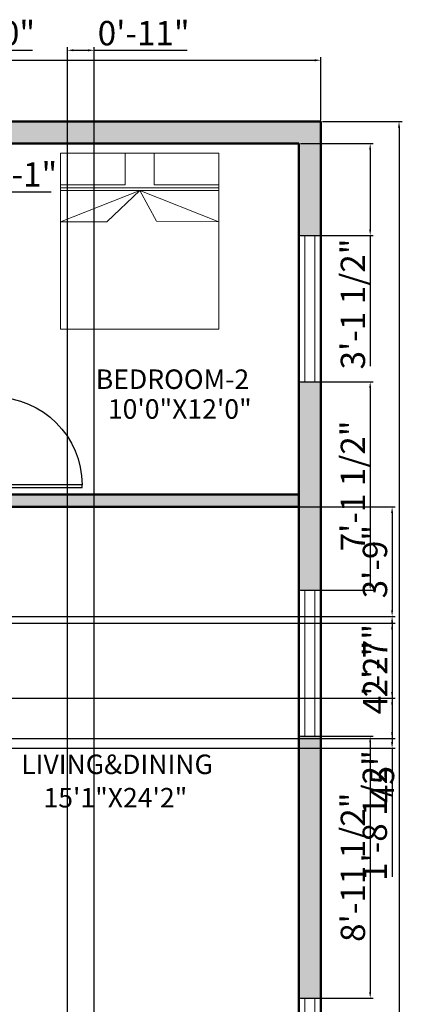
# Model space of a CAD drawing. Units: inches. Extents: x 2719 to 3167, y 1639 to 2327.
# Tile 4 of 4: x 3005 to 3167, y 1881 to 2285. Entities that reach past the tile are written whole.
import ezdxf

# ---------------------------------------------------------------- set-up
doc = ezdxf.new("R2010")
doc.units = ezdxf.units.IN
for name, color, linetype, lineweight in [('A-ANNO-DIMS', 121, 'Continuous', 18), ('A-AREA-IDEN', 121, 'Continuous', 18), ('A-DOOR', 50, 'Continuous', 25), ('A-FURN', 211, 'Continuous', 18), ('A-GLAZ', 191, 'Continuous', 18), ('A-WALL', 7, 'Continuous', 50)]:
    doc.layers.add(name, color=color, linetype=linetype, lineweight=lineweight)
doc.layers.add('A-WALL-PATT', color=251, linetype='Continuous', lineweight=13, true_color=0x636466)
doc.styles.get("Standard").update_dxf_attribs({"font": 'arial.ttf'})
doc.dimstyles.new('ISO-25', dxfattribs={"dimtxt": 10, "dimasz": 2.5, "dimexe": 1.25, "dimexo": 0.625, "dimtad": 1, "dimdec": 0, "dimlunit": 3, "dimtxsty": 'Standard', "dimcen": 2.5, "dimadec": 0, "dimazin": 0, "dimtfac": 1, "dimtdec": 0, "dimtmove": 0, "dimatfit": 3, "dimfxl": 1, "dimarcsym": 0})

# ---------------------------------------------------------------- blocks, each defined once
blk = doc.blocks.new('*D1')
at = {"layer": 'A-ANNO-DIMS', "color": 0, "lineweight": -2, "transparency": 16777216}
for p, q in [((2768.8, 2244.06), (2768.8, 2269.84)), ((3128.8, 2244.06), (3128.8, 2269.84)), ((2771.3, 2268.59), (3126.3, 2268.59))]:
    blk.add_line(p, q, dxfattribs=at)
at = {"layer": 'A-ANNO-DIMS', "color": 0, "transparency": 16777216}
for points in [[(2771.3, 2269.01), (2771.3, 2268.17), (2768.8, 2268.59)], [(3126.3, 2269.01), (3126.3, 2268.17), (3128.8, 2268.59)]]:
    blk.add_solid(points, dxfattribs=at)
at = {"layer": 'Defpoints', "color": 0, "transparency": 16777216}
for p in [(3128.8, 2268.59), (2768.8, 2243.44), (3128.8, 2243.44)]:
    blk.add_point(p, dxfattribs=at)
at = {"layer": 'A-ANNO-DIMS', "color": 0, "transparency": 16777216, "insert": (2948.8, 2274.32), "char_height": 10, "attachment_point": 5}
blk.add_mtext("30'", dxfattribs=at)
blk = doc.blocks.new('*D2')
at = {"layer": 'A-ANNO-DIMS', "color": 0, "lineweight": -2, "transparency": 16777216}
for p, q in [((3129.42, 2243.44), (3162.14, 2243.44)), ((3160.89, 2240.94), (3160.89, 1705.94)), ((3129.42, 1703.44), (3162.14, 1703.44))]:
    blk.add_line(p, q, dxfattribs=at)
at = {"layer": 'A-ANNO-DIMS', "color": 0, "transparency": 16777216}
for points in [[(3160.47, 2240.94), (3161.31, 2240.94), (3160.89, 2243.44)], [(3160.47, 1705.94), (3161.31, 1705.94), (3160.89, 1703.44)]]:
    blk.add_solid(points, dxfattribs=at)
at = {"layer": 'Defpoints', "color": 0, "transparency": 16777216}
for p in [(3128.8, 2243.44), (3128.8, 1703.44), (3160.89, 1703.44)]:
    blk.add_point(p, dxfattribs=at)
at = {"layer": 'A-ANNO-DIMS', "color": 0, "transparency": 16777216, "insert": (3155.18, 1973.44), "char_height": 10, "attachment_point": 5, "rotation": 90}
blk.add_mtext("45'", dxfattribs=at)
blk = doc.blocks.new('BED-DOUBLE')
for p, q in [((0, 57.96), (64.91, 57.96)), ((0, 56.96), (64.91, 56.96)), ((32.46, 56.96), (0, 44.1)), ((32.46, 56.96), (18.94, 44.05)), ((32.46, 56.96), (64.91, 44.04)), ((32.46, 56.96), (39.4, 44.29)), ((18.94, 44.05), (0, 44.05)), ((39.4, 44.29), (64.91, 44.04))]:
    blk.add_line(p, q)
for points in [[(0, 72.15), (64.91, 72.15), (64.91, 0), (0, 0)], [(0, 72.15), (26.55, 72.15), (26.55, 59.27), (0, 59.27)], [(38.37, 72.15), (64.91, 72.15), (64.91, 59.27), (38.37, 59.27)]]:
    blk.add_lwpolyline(points, close=True)
blk = doc.blocks.new('WIN-60IN')
for p, q in [((9, 60), (0, 60)), ((2.5, 60), (2.5, 0)), ((6.5, 60), (6.5, 0)), ((9, 0), (0, 0))]:
    blk.add_line(p, q)
blk = doc.blocks.new('DOOR-36IN-QUARTER-SWING')
for p, q in [((0, 0), (0, 1)), ((0, 1), (36, 1)), ((36, 0), (0, 0)), ((36, 1), (36, 0))]:
    blk.add_line(p, q)
blk.add_arc((36, 1), 36, 90, 180)
blk = doc.blocks.new('*D18')
at = {"layer": 'A-ANNO-DIMS', "color": 0, "lineweight": -2, "transparency": 16777216}
for p, q in [((2955.97, 2244.06), (2955.97, 2273.94)), ((2979.97, 2244.06), (2979.97, 2273.94)), ((2958.47, 2272.69), (2977.47, 2272.69)), ((2979.97, 2272.69), (3010.48, 2272.69))]:
    blk.add_line(p, q, dxfattribs=at)
at = {"layer": 'A-ANNO-DIMS', "color": 0, "transparency": 16777216}
for points in [[(2958.47, 2273.1), (2958.47, 2272.27), (2955.97, 2272.69)], [(2977.47, 2273.1), (2977.47, 2272.27), (2979.97, 2272.69)]]:
    blk.add_solid(points, dxfattribs=at)
at = {"layer": 'Defpoints', "color": 0, "transparency": 16777216}
for p in [(2979.97, 2272.69), (2955.97, 2243.44), (2979.97, 2243.44)]:
    blk.add_point(p, dxfattribs=at)
at = {"layer": 'A-ANNO-DIMS', "color": 0, "transparency": 16777216, "insert": (2996.48, 2278.42), "char_height": 10, "attachment_point": 5}
blk.add_mtext('2\'-0"', dxfattribs=at)
blk = doc.blocks.new('*D23')
at = {"layer": 'A-ANNO-DIMS', "color": 0, "lineweight": -2, "transparency": 16777216}
for p, q in [((3120.42, 2234.44), (3150.3, 2234.44)), ((3149.05, 2231.94), (3149.05, 2199.22)), ((3120.42, 2196.72), (3150.3, 2196.72)), ((3149.05, 2196.72), (3149.05, 2143.09))]:
    blk.add_line(p, q, dxfattribs=at)
at = {"layer": 'A-ANNO-DIMS', "color": 0, "transparency": 16777216}
for points in [[(3148.63, 2231.94), (3149.46, 2231.94), (3149.05, 2234.44)], [(3148.63, 2199.22), (3149.46, 2199.22), (3149.05, 2196.72)]]:
    blk.add_solid(points, dxfattribs=at)
at = {"layer": 'Defpoints', "color": 0, "transparency": 16777216}
for p in [(3119.8, 2234.44), (3119.8, 2196.72), (3149.05, 2196.72)]:
    blk.add_point(p, dxfattribs=at)
at = {"layer": 'A-ANNO-DIMS', "color": 0, "transparency": 16777216, "insert": (3143.25, 2168.65), "char_height": 10, "attachment_point": 5, "rotation": 90}
blk.add_mtext('3\'-1 1/2"', dxfattribs=at)
blk = doc.blocks.new('*D24')
at = {"layer": 'A-ANNO-DIMS', "color": 0, "lineweight": -2, "transparency": 16777216}
for p, q in [((3120.42, 2136.72), (3150.3, 2136.72)), ((3149.05, 2134.22), (3149.05, 2053.83)), ((3120.42, 2051.33), (3150.3, 2051.33))]:
    blk.add_line(p, q, dxfattribs=at)
at = {"layer": 'A-ANNO-DIMS', "color": 0, "transparency": 16777216}
for points in [[(3148.63, 2134.22), (3149.46, 2134.22), (3149.05, 2136.72)], [(3148.63, 2053.83), (3149.46, 2053.83), (3149.05, 2051.33)]]:
    blk.add_solid(points, dxfattribs=at)
at = {"layer": 'Defpoints', "color": 0, "transparency": 16777216}
for p in [(3119.8, 2136.72), (3119.8, 2051.33), (3149.05, 2051.33)]:
    blk.add_point(p, dxfattribs=at)
at = {"layer": 'A-ANNO-DIMS', "color": 0, "transparency": 16777216, "insert": (3143.25, 2094.02), "char_height": 10, "attachment_point": 5, "rotation": 90}
blk.add_mtext('7\'-1 1/2"', dxfattribs=at)
blk = doc.blocks.new('*D25')
at = {"layer": 'A-ANNO-DIMS', "color": 0, "lineweight": -2, "transparency": 16777216}
for p, q in [((3120.42, 1991.33), (3150.3, 1991.33)), ((3149.05, 1988.83), (3149.05, 1886.45)), ((3120.42, 1883.95), (3150.3, 1883.95))]:
    blk.add_line(p, q, dxfattribs=at)
at = {"layer": 'A-ANNO-DIMS', "color": 0, "transparency": 16777216}
for points in [[(3148.63, 1988.83), (3149.46, 1988.83), (3149.05, 1991.33)], [(3148.63, 1886.45), (3149.46, 1886.45), (3149.05, 1883.95)]]:
    blk.add_solid(points, dxfattribs=at)
at = {"layer": 'Defpoints', "color": 0, "transparency": 16777216}
for p in [(3119.8, 1991.33), (3119.8, 1883.95), (3149.05, 1883.95)]:
    blk.add_point(p, dxfattribs=at)
at = {"layer": 'A-ANNO-DIMS', "color": 0, "transparency": 16777216, "insert": (3143.25, 1937.64), "char_height": 10, "attachment_point": 5, "rotation": 90}
blk.add_mtext('8\'-11 1/2"', dxfattribs=at)
blk = doc.blocks.new('*D29')
at = {"layer": 'A-ANNO-DIMS', "color": 0, "lineweight": -2, "transparency": 16777216}
for p, q in [((2939.42, 2040.53), (3159.3, 2040.53)), ((3158.05, 2038.03), (3158.05, 1992.94)), ((2939.42, 1990.44), (3159.3, 1990.44))]:
    blk.add_line(p, q, dxfattribs=at)
at = {"layer": 'A-ANNO-DIMS', "color": 0, "transparency": 16777216}
for points in [[(3157.63, 2038.03), (3158.46, 2038.03), (3158.05, 2040.53)], [(3157.63, 1992.94), (3158.46, 1992.94), (3158.05, 1990.44)]]:
    blk.add_solid(points, dxfattribs=at)
at = {"layer": 'Defpoints', "color": 0, "transparency": 16777216}
for p in [(2938.8, 2040.53), (2938.8, 1990.44), (3158.05, 1990.44)]:
    blk.add_point(p, dxfattribs=at)
at = {"layer": 'A-ANNO-DIMS', "color": 0, "transparency": 16777216, "insert": (3152.4, 2015.48), "char_height": 10, "attachment_point": 5, "rotation": 90}
blk.add_mtext('4\'-2"', dxfattribs=at)
blk = doc.blocks.new('*D30')
at = {"layer": 'A-ANNO-DIMS', "color": 0, "lineweight": -2, "transparency": 16777216}
for p, q in [((2934.42, 2085.44), (3159.3, 2085.44)), ((3158.05, 2082.94), (3158.05, 2043.03)), ((2934.42, 2040.53), (3159.3, 2040.53))]:
    blk.add_line(p, q, dxfattribs=at)
at = {"layer": 'A-ANNO-DIMS', "color": 0, "transparency": 16777216}
for points in [[(3157.63, 2082.94), (3158.46, 2082.94), (3158.05, 2085.44)], [(3157.63, 2043.03), (3158.46, 2043.03), (3158.05, 2040.53)]]:
    blk.add_solid(points, dxfattribs=at)
at = {"layer": 'Defpoints', "color": 0, "transparency": 16777216}
for p in [(2933.8, 2085.44), (2933.8, 2040.53), (3158.05, 2040.53)]:
    blk.add_point(p, dxfattribs=at)
at = {"layer": 'A-ANNO-DIMS', "color": 0, "transparency": 16777216, "insert": (3152.31, 2062.98), "char_height": 10, "attachment_point": 5, "rotation": 90}
blk.add_mtext('3\'-9"', dxfattribs=at)
blk = doc.blocks.new('*D34')
at = {"layer": 'A-ANNO-DIMS', "color": 0, "lineweight": -2, "transparency": 16777216}
for p, q in [((2800.47, 2037.74), (3159.3, 2037.74)), ((3158.05, 2035.24), (3158.05, 2009.46)), ((2800.47, 2006.96), (3159.3, 2006.96))]:
    blk.add_line(p, q, dxfattribs=at)
at = {"layer": 'A-ANNO-DIMS', "color": 0, "transparency": 16777216}
for points in [[(3157.63, 2035.24), (3158.46, 2035.24), (3158.05, 2037.74)], [(3157.63, 2009.46), (3158.46, 2009.46), (3158.05, 2006.96)]]:
    blk.add_solid(points, dxfattribs=at)
at = {"layer": 'Defpoints', "color": 0, "transparency": 16777216}
for p in [(2799.85, 2037.74), (2799.85, 2006.96), (3158.05, 2006.96)]:
    blk.add_point(p, dxfattribs=at)
at = {"layer": 'A-ANNO-DIMS', "color": 0, "transparency": 16777216, "insert": (3152.4, 2022.35), "char_height": 10, "attachment_point": 5, "rotation": 90}
blk.add_mtext('2\'-7"', dxfattribs=at)
blk = doc.blocks.new('*D35')
at = {"layer": 'A-ANNO-DIMS', "color": 0, "lineweight": -2, "transparency": 16777216}
for p, q in [((2800.47, 2006.96), (3159.3, 2006.96)), ((3158.05, 2004.46), (3158.05, 1988.94)), ((2806.13, 1986.44), (3159.3, 1986.44)), ((3158.05, 1986.44), (3158.05, 1933.74))]:
    blk.add_line(p, q, dxfattribs=at)
at = {"layer": 'A-ANNO-DIMS', "color": 0, "transparency": 16777216}
for points in [[(3157.63, 2004.46), (3158.46, 2004.46), (3158.05, 2006.96)], [(3157.63, 1988.94), (3158.46, 1988.94), (3158.05, 1986.44)]]:
    blk.add_solid(points, dxfattribs=at)
at = {"layer": 'Defpoints', "color": 0, "transparency": 16777216}
for p in [(2799.85, 2006.96), (2805.5, 1986.44), (3158.05, 1986.44)]:
    blk.add_point(p, dxfattribs=at)
at = {"layer": 'A-ANNO-DIMS', "color": 0, "transparency": 16777216, "insert": (3152.25, 1958.84), "char_height": 10, "attachment_point": 5, "rotation": 90}
blk.add_mtext('1\'-8 1/2"', dxfattribs=at)
blk = doc.blocks.new('*D46')
at = {"layer": 'A-ANNO-DIMS', "color": 0, "lineweight": -2, "transparency": 16777216}
for p, q in [((3024.8, 1791.06), (3024.8, 2273.94)), ((3035.8, 1791.06), (3035.8, 2273.94)), ((3027.3, 2272.69), (3033.3, 2272.69)), ((3035.8, 2272.69), (3073.9, 2272.69))]:
    blk.add_line(p, q, dxfattribs=at)
at = {"layer": 'A-ANNO-DIMS', "color": 0, "transparency": 16777216}
for points in [[(3027.3, 2273.1), (3027.3, 2272.27), (3024.8, 2272.69)], [(3033.3, 2273.1), (3033.3, 2272.27), (3035.8, 2272.69)]]:
    blk.add_solid(points, dxfattribs=at)
at = {"layer": 'Defpoints', "color": 0, "transparency": 16777216}
for p in [(3035.8, 2272.69), (3024.8, 1790.44), (3035.8, 1790.44)]:
    blk.add_point(p, dxfattribs=at)
at = {"layer": 'A-ANNO-DIMS', "color": 0, "transparency": 16777216, "insert": (3056.1, 2278.42), "char_height": 10, "attachment_point": 5}
blk.add_mtext('0\'-11"', dxfattribs=at)
blk = doc.blocks.new('*D57')
at = {"layer": 'A-ANNO-DIMS', "color": 0, "lineweight": -2, "transparency": 16777216}
for p, q in [((2959.06, 2214.46), (2956.56, 2214.46)), ((2961.56, 2214.46), (2974.39, 2214.46)), ((3018.1, 2214.46), (2976.89, 2214.46))]:
    blk.add_line(p, q, dxfattribs=at)
at = {"layer": 'A-ANNO-DIMS', "color": 0, "transparency": 16777216}
for points in [[(2959.06, 2214.88), (2959.06, 2214.05), (2961.56, 2214.46)], [(2976.89, 2214.88), (2976.89, 2214.05), (2974.39, 2214.46)]]:
    blk.add_solid(points, dxfattribs=at)
at = {"layer": 'Defpoints', "color": 0, "transparency": 16777216}
for p in [(2961.56, 2214.46), (2974.39, 2214.46)]:
    blk.add_point(p, dxfattribs=at)
at = {"layer": 'A-ANNO-DIMS', "color": 0, "transparency": 16777216, "insert": (2998.74, 2220.47), "char_height": 10, "attachment_point": 5, "rotation": 359.9976}
blk.add_mtext('∅1\'-1"', dxfattribs=at)

msp = doc.modelspace()

# ---------------------------------------------------------------- hatches: boundary and pattern name
at = {"layer": 'A-WALL-PATT'}
h = msp.add_hatch(color=256, dxfattribs=at)
h.dxf.hatch_style = 1
h.paths.add_polyline_path([(3128.8, 2243.44), (2979.97, 2243.44), (2979.97, 2234.44), (3119.8, 2234.44), (3119.8, 2196.72), (3128.8, 2196.72)])
h = msp.add_hatch(color=256, dxfattribs=at)
h.dxf.hatch_style = 1
h.paths.add_polyline_path([(3128.8, 2136.72), (3119.8, 2136.72), (3119.8, 2051.33), (3128.8, 2051.33)])
h = msp.add_hatch(color=256, dxfattribs=at)
h.dxf.hatch_style = 1
h.paths.add_polyline_path([(3119.8, 2090.44), (2999.8, 2090.44), (2999.8, 2093.44), (2994.8, 2093.44), (2994.8, 2090.44), (2994.8, 2085.44), (3119.8, 2085.44)])
h = msp.add_hatch(color=256, dxfattribs=at)
h.dxf.hatch_style = 1
h.paths.add_polyline_path([(3128.8, 1991.33), (3119.8, 1991.33), (3119.8, 1883.95), (3128.8, 1883.95)])

# ---------------------------------------------------------------- linework, layer by layer
at = {"layer": 'A-WALL'}
for p, q in [((2777.8, 2234.44), (3119.8, 2234.44)), ((3119.8, 2234.44), (3119.8, 1712.44)), ((2999.8, 2090.44), (3119.8, 2090.44)), ((2994.8, 2085.44), (3119.8, 2085.44))]:
    msp.add_line(p, q, dxfattribs=at)
msp.add_lwpolyline([(2941.8, 1703.44), (2768.8, 1703.44), (2768.8, 2243.44), (3128.8, 2243.44), (3128.8, 1703.44), (2989.8, 1703.44)], dxfattribs=at)

# ---------------------------------------------------------------- block references
at = {"layer": 'A-DOOR', "extrusion": (0, 0, -1), "zscale": -1}
msp.add_blockref('DOOR-36IN-QUARTER-SWING', (-3030.8, 2093.44), dxfattribs=at)
at = {"layer": 'A-FURN'}
msp.add_blockref('BED-DOUBLE', (3022, 2158.28), dxfattribs=at)
at = {"layer": 'A-GLAZ', "rotation": 180}
for p in [(3128.8, 2196.72), (3128.8, 2051.33)]:
    msp.add_blockref('WIN-60IN', p, dxfattribs=at)
at = {"layer": 'A-GLAZ'}
msp.add_blockref('WIN-60IN', (3119.8, 1823.95), dxfattribs=at)

# ---------------------------------------------------------------- texts
at = {"layer": 'A-AREA-IDEN'}
for tag, p in [('BEDROOM-2', (3036.45, 2133.79)), ('10\'0"X12\'0"', (3041.41, 2121.58)), ('LIVING&DINING', (3005.85, 1975.85)), ('15\'1"X24\'2"', (3014.99, 1962.15))]:
    msp.add_attdef(tag, p, '', height=8, dxfattribs=at)

# ---------------------------------------------------------------- dimensions: what is measured, and where the dimension line sits
at = {"layer": 'A-ANNO-DIMS'}
for base, p1, p2, override, picture, middle in [((2979.97, 2272.69), (2955.97, 2243.44), (2979.97, 2243.44), {"dimdec": 1, "dimlfac": 1, "dimrnd": 0, "dimzin": 1, "dimdsep": 46, "dimlunit": 4, "dimfrac": 2}, '*D18', (2996.48, 2278.42)), ((3035.8, 2272.69), (3024.8, 1790.44), (3035.8, 1790.44), {"dimdec": 1, "dimlfac": 1, "dimrnd": 0, "dimzin": 1, "dimdsep": 46, "dimlunit": 4, "dimfrac": 2}, '*D46', (3056.1, 2278.42)), ((3128.8, 2268.59), (2768.8, 2243.44), (3128.8, 2243.44), {"dimclrd": 0, "dimclre": 0, "dimclrt": 0}, '*D1', (2948.8, 2274.32))]:
    dim = msp.add_linear_dim(base=base, p1=p1, p2=p2, dimstyle='ISO-25', override=override, dxfattribs=at)
    dim.commit()
    dim.dimension.update_dxf_attribs({"geometry": picture, "text_midpoint": middle})
for base, p1, p2, angle, override, picture, middle in [((3160.89, 1703.44), (3128.8, 2243.44), (3128.8, 1703.44), 90, {"dimclrd": 0, "dimclre": 0, "dimclrt": 0}, '*D2', (3155.18, 1973.44)), ((3149.05, 2196.72), (3119.8, 2234.44), (3119.8, 2196.72), 270, {"dimdec": 1, "dimlfac": 1, "dimrnd": 0, "dimzin": 1, "dimdsep": 46, "dimlunit": 4, "dimfrac": 2}, '*D23', (3143.25, 2168.65)), ((3149.05, 2051.33), (3119.8, 2136.72), (3119.8, 2051.33), 270, {"dimdec": 1, "dimlfac": 1, "dimrnd": 0, "dimzin": 1, "dimdsep": 46, "dimlunit": 4, "dimfrac": 2}, '*D24', (3143.25, 2094.02)), ((3158.05, 2040.53), (2933.8, 2085.44), (2933.8, 2040.53), 90, {"dimdec": 1, "dimlfac": 1, "dimrnd": 0, "dimzin": 1, "dimdsep": 46, "dimlunit": 4, "dimfrac": 2}, '*D30', (3152.31, 2062.98)), ((3158.05, 1990.44), (2938.8, 2040.53), (2938.8, 1990.44), 90, {"dimdec": 1, "dimlfac": 1, "dimrnd": 0, "dimzin": 1, "dimdsep": 46, "dimlunit": 4, "dimfrac": 2}, '*D29', (3152.4, 2015.48)), ((3158.05, 2006.96), (2799.85, 2037.74), (2799.85, 2006.96), 90, {"dimdec": 1, "dimlfac": 1, "dimrnd": 0, "dimzin": 1, "dimdsep": 46, "dimlunit": 4, "dimfrac": 2}, '*D34', (3152.4, 2022.35)), ((3158.05, 1986.44), (2799.85, 2006.96), (2805.5, 1986.44), 90, {"dimdec": 1, "dimlfac": 1, "dimrnd": 0, "dimzin": 1, "dimdsep": 46, "dimlunit": 4, "dimfrac": 2}, '*D35', (3152.25, 1958.84)), ((3149.05, 1883.95), (3119.8, 1991.33), (3119.8, 1883.95), 270, {"dimdec": 1, "dimlfac": 1, "dimrnd": 0, "dimzin": 1, "dimdsep": 46, "dimlunit": 4, "dimfrac": 2}, '*D25', (3143.25, 1937.64))]:
    dim = msp.add_linear_dim(base=base, p1=p1, p2=p2, angle=angle, dimstyle='ISO-25', override=override, dxfattribs=at)
    dim.commit()
    dim.dimension.update_dxf_attribs({"geometry": picture, "text_midpoint": middle})
dim = msp.add_diameter_dim_2p(p1=(2961.56, 2214.46), p2=(2974.39, 2214.46), dimstyle='ISO-25', override={"dimdec": 1, "dimlfac": 1, "dimrnd": 0, "dimzin": 1, "dimdsep": 46, "dimlunit": 4, "dimfrac": 2}, dxfattribs=at)
dim.commit()
dim.dimension.update_dxf_attribs({"geometry": '*D57', "text_midpoint": (2998.74, 2214.46)})

doc.saveas('drawing.dxf')
